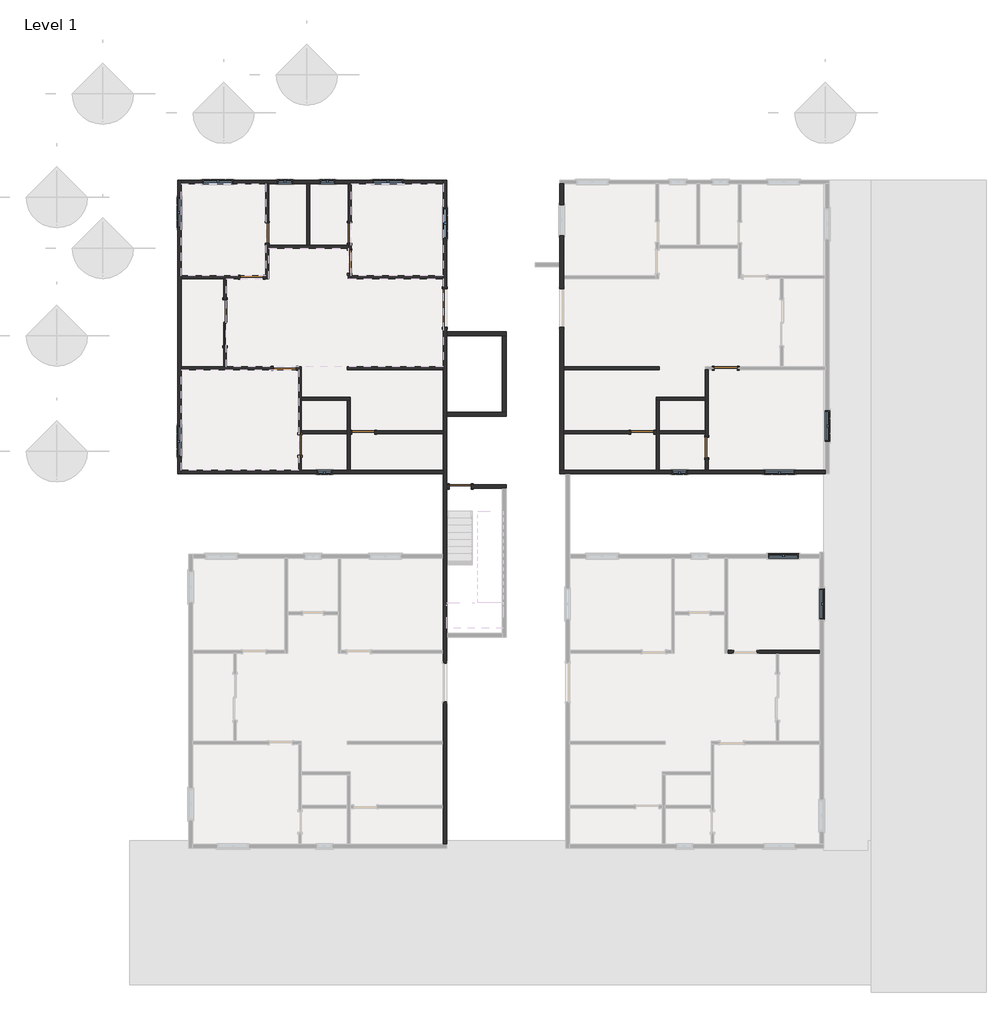
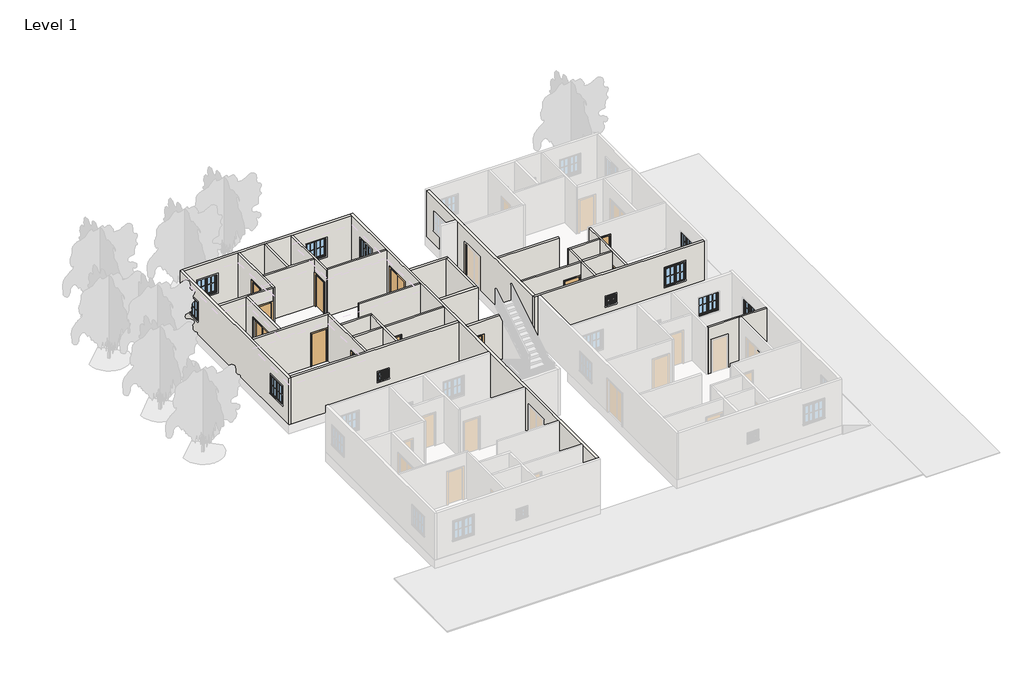
# One storey, part 2 of 7: 29 walls, 13 doors, 13 windows.
# Revit data of these elements (continued)
# Element 43 (IfcWindow, "Window-Casement-Double : 24\" x 24\"") (continued)
#   Exterior Wall Closure = 0' - 1 1/4"
#   Interior Trim Visibility = yes
#   Exterior Trim Visibility = yes
#   Phase Created = New Construction
#   Materials on its faces: "Wood - Stained", "Glass", "Clad - White"
# Element 44 (IfcWindow, "Window-Casement-Double : 24\" x 24\"")
#   Mark = "24"
#   Window Inset = 0' - 0"
#   Interior Wall Closure = 0' - 2 1/4"
#   Frame Extension = 0' - 0 1/4"
#   Exterior Wall Closure = 0' - 1 1/4"
#   Interior Trim Visibility = yes
#   Exterior Trim Visibility = yes
#   Phase Created = New Construction
#   Materials on its faces: "Wood - Stained", "Glass", "Clad - White"
# Element 45 (IfcWindow, "Window-Casement-Double : 24\" x 24\"")
#   Mark = "25"
#   Window Inset = 0' - 0"
#   Interior Wall Closure = 0' - 2 1/4"
#   Frame Extension = 0' - 0 1/4"
#   Exterior Wall Closure = 0' - 1 1/4"
#   Interior Trim Visibility = yes
#   Exterior Trim Visibility = yes
#   Phase Created = New Construction
#   Materials on its faces: "Wood - Stained", "Glass", "Clad - White"
# Element 46 (IfcWindow, "Window-Casement-Double : 24\" x 24\"")
#   Mark = "30"
#   Window Inset = 0' - 0"
#   Interior Wall Closure = 0' - 2 1/4"
#   Frame Extension = 0' - 0 1/4"
#   Exterior Wall Closure = 0' - 1 1/4"
#   Interior Trim Visibility = yes
#   Exterior Trim Visibility = yes
#   Phase Created = New Construction
#   Materials on its faces: "Wood - Stained", "Glass", "Clad - White"
# Element 47 (IfcWindow, "Window-Casement-Double : 48\" x 48\"")
#   Mark = "1"
#   Window Inset = 0' - 0"
#   Interior Wall Closure = 0' - 2 1/4"
#   Frame Extension = 0' - 0 1/4"
#   Exterior Wall Closure = 0' - 1 1/4"
#   Interior Trim Visibility = yes
#   Exterior Trim Visibility = yes
#   Phase Created = New Construction
#   Materials on its faces: "Wood - Stained", "Glass", "Clad - White"
# Element 48 (IfcWindow, "Window-Casement-Double : 48\" x 48\"")
#   Mark = "2"
#   Window Inset = 0' - 0"
#   Interior Wall Closure = 0' - 2 1/4"
#   Frame Extension = 0' - 0 1/4"
#   Exterior Wall Closure = 0' - 1 1/4"
#   Interior Trim Visibility = yes
#   Exterior Trim Visibility = yes
#   Phase Created = New Construction
#   Materials on its faces: "Wood - Stained", "Glass", "Clad - White"
# Element 49 (IfcWindow, "Window-Casement-Double : 48\" x 48\"")
#   Mark = "3"
#   Window Inset = 0' - 0"
#   Interior Wall Closure = 0' - 2 1/4"
#   Frame Extension = 0' - 0 1/4"
#   Exterior Wall Closure = 0' - 1 1/4"
#   Interior Trim Visibility = yes
#   Exterior Trim Visibility = yes
#   Phase Created = New Construction
#   Materials on its faces: "Wood - Stained", "Glass", "Clad - White"
# Element 50 (IfcWindow, "Window-Casement-Double : 48\" x 48\"")
#   Mark = "4"
#   Window Inset = 0' - 0"
#   Interior Wall Closure = 0' - 2 1/4"
#   Frame Extension = 0' - 0 1/4"
#   Exterior Wall Closure = 0' - 1 1/4"
#   Interior Trim Visibility = yes
#   Exterior Trim Visibility = yes
#   Phase Created = New Construction
#   Materials on its faces: "Wood - Stained", "Glass", "Clad - White"
# Element 51 (IfcWindow, "Window-Casement-Double : 48\" x 48\"")
#   Mark = "5"
#   Window Inset = 0' - 0"
#   Interior Wall Closure = 0' - 2 1/4"
#   Frame Extension = 0' - 0 1/4"
#   Exterior Wall Closure = 0' - 1 1/4"
#   Interior Trim Visibility = yes
#   Exterior Trim Visibility = yes
#   Phase Created = New Construction
#   Materials on its faces: "Wood - Stained", "Glass", "Clad - White"
# Element 52 (IfcWindow, "Window-Casement-Double : 48\" x 48\"")
#   Mark = "10"
#   Window Inset = 0' - 0"
#   Interior Wall Closure = 0' - 2 1/4"
#   Frame Extension = 0' - 0 1/4"
#   Exterior Wall Closure = 0' - 1 1/4"
#   Interior Trim Visibility = yes
#   Exterior Trim Visibility = yes
#   Phase Created = New Construction
#   Materials on its faces: "Wood - Stained", "Glass", "Clad - White"
# Element 53 (IfcWindow, "Window-Casement-Double : 48\" x 48\"")
#   Mark = "11"
#   Window Inset = 0' - 0"
#   Interior Wall Closure = 0' - 2 1/4"
#   Frame Extension = 0' - 0 1/4"
#   Exterior Wall Closure = 0' - 1 1/4"
#   Interior Trim Visibility = yes
#   Exterior Trim Visibility = yes
#   Phase Created = New Construction
#   Materials on its faces: "Wood - Stained", "Glass", "Clad - White"
# Element 54 (IfcWindow, "Window-Casement-Double : 48\" x 48\"")
#   Mark = "19"
#   Window Inset = 0' - 0"
#   Interior Wall Closure = 0' - 2 1/4"
#   Frame Extension = 0' - 0 1/4"
#   Exterior Wall Closure = 0' - 1 1/4"
#   Interior Trim Visibility = yes
#   Exterior Trim Visibility = yes
#   Phase Created = New Construction
#   Materials on its faces: "Wood - Stained", "Glass", "Clad - White"
# Element 55 (IfcWindow, "Window-Casement-Double : 48\" x 48\"")
#   Mark = "20"
#   Window Inset = 0' - 0"
#   Interior Wall Closure = 0' - 2 1/4"
#   Frame Extension = 0' - 0 1/4"
#   Exterior Wall Closure = 0' - 1 1/4"
#   Interior Trim Visibility = yes
#   Exterior Trim Visibility = yes
#   Phase Created = New Construction
#   Materials on its faces: "Wood - Stained", "Glass", "Clad - White"
# Materials
#   "Wood - Birch - Solid Stained Light Low Gloss": class "Wood", colour RGB 210 159 95, transparency 0, Cost = 0
#   "Paint - Sienna": colour RGB 118 70 51, transparency 0, Cost = 0
#   "Glass": class "Glass", colour RGB 0 128 192, transparency 0.75, Description = "Soda Lime Glass", Cost = 0
#   "Door - Panel": class "Wood", colour RGB 210 159 95, transparency 0, Cost = 0
#   "Door - Frame": colour RGB 118 70 51, transparency 0, Cost = 0
#   "4.5\" WALL": class "Generic", colour RGB 120 120 120, transparency 0, Cost = 0
#   "6\" WALL": class "Generic", colour RGB 120 120 120, transparency 0, Cost = 0
#   "Wood - Stained": class "Wood", colour RGB 224 178 126, transparency 0, Cost = 0
#   "Clad - White": class "Wood", colour RGB 242 242 238, transparency 0, Cost = 0
